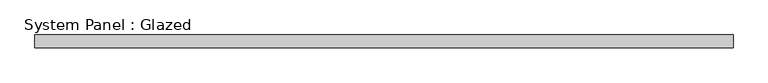
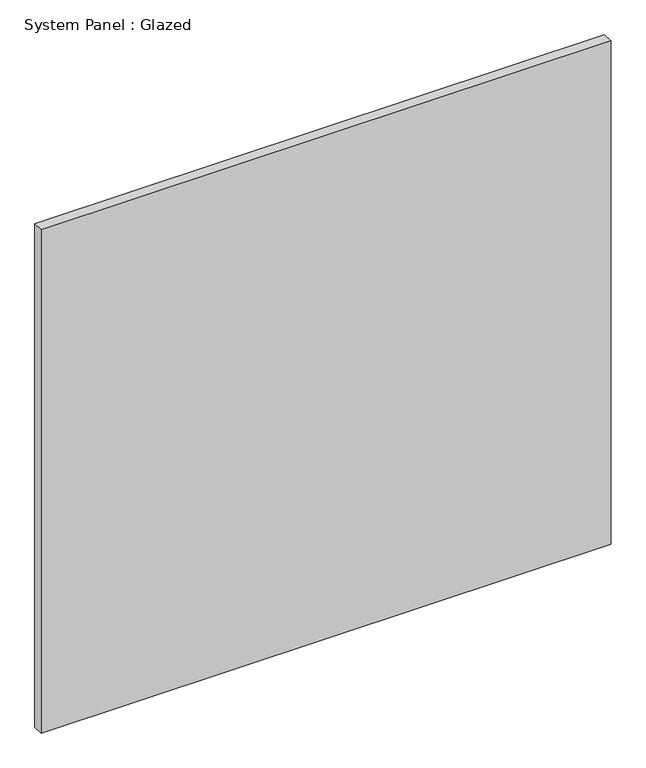
"""IFC4 building model written with IfcOpenShell, lengths in millimetres: plate geometry, System Panel : Glazed."""

from ifc_helpers import new_model, si_unit, origin, origin_with_axes, place, context, project, spatial, polyline, outline, extrude, source, transform, mapped, element, save


def system_panel_glazed_fa23d52e(model_context):
    return source(origin(), model_context, "Body", "SweptSolid", [
        extrude(outline(polyline([(683.6833332, 19.05), (-683.6833332, 19.05), (-683.6833332, 44.45), (683.6833332, 44.45), (683.6833332, 19.05)])), origin_with_axes(), (0.0, 0.0, 1.0), 1276.35),
    ])


if __name__ == "__main__":
    model = new_model("IFC4")
    model_context = context("Model", 3, world=origin())
    ifc_project = project(units=[si_unit("LENGTHUNIT", "METRE", prefix="MILLI")], contexts=[model_context])
    site = spatial("IfcSite", under=ifc_project)
    building = spatial("IfcBuilding", under=site)
    placement = place(None, origin())
    system_panel_glazed_shape = system_panel_glazed_fa23d52e(model_context)
    element("IfcPlate", 1, ObjectType="System Panel : Glazed", at=placement, inside=building, context=model_context, shape_type="MappedRepresentation", body=[
        mapped(system_panel_glazed_shape, transform((0.0, 0.0, 0.0), x_axis=(1.0, 0.0, 0.0), y_axis=(0.0, 1.0, 0.0), z_axis=(0.0, 0.0, 1.0))),
    ])
    save(model, "model.ifc")

# Revit data of these elements
# Type "System Panel : Glazed"
#   Construction Type Id = "GSP4R"
#   Analytic Construction = "1/8 in Pilkington single glazing"
#   Visual Light Transmittance = 0.9
#   Solar Heat Gain Coefficient = 0.86
#   Heat Transfer Coefficient (U) = 1.18115 BTU/(h·ft²·°F)
#   Define Thermal Properties by = 1
# Element 1 (IfcPlate, "System Panel : Glazed")
#   Materials on its faces: "Glass"
# Materials
#   "Glass": class "Glass", colour RGB 0 128 192, transparency 0.75, Description = "Soda Lime Glass", Cost = 0
